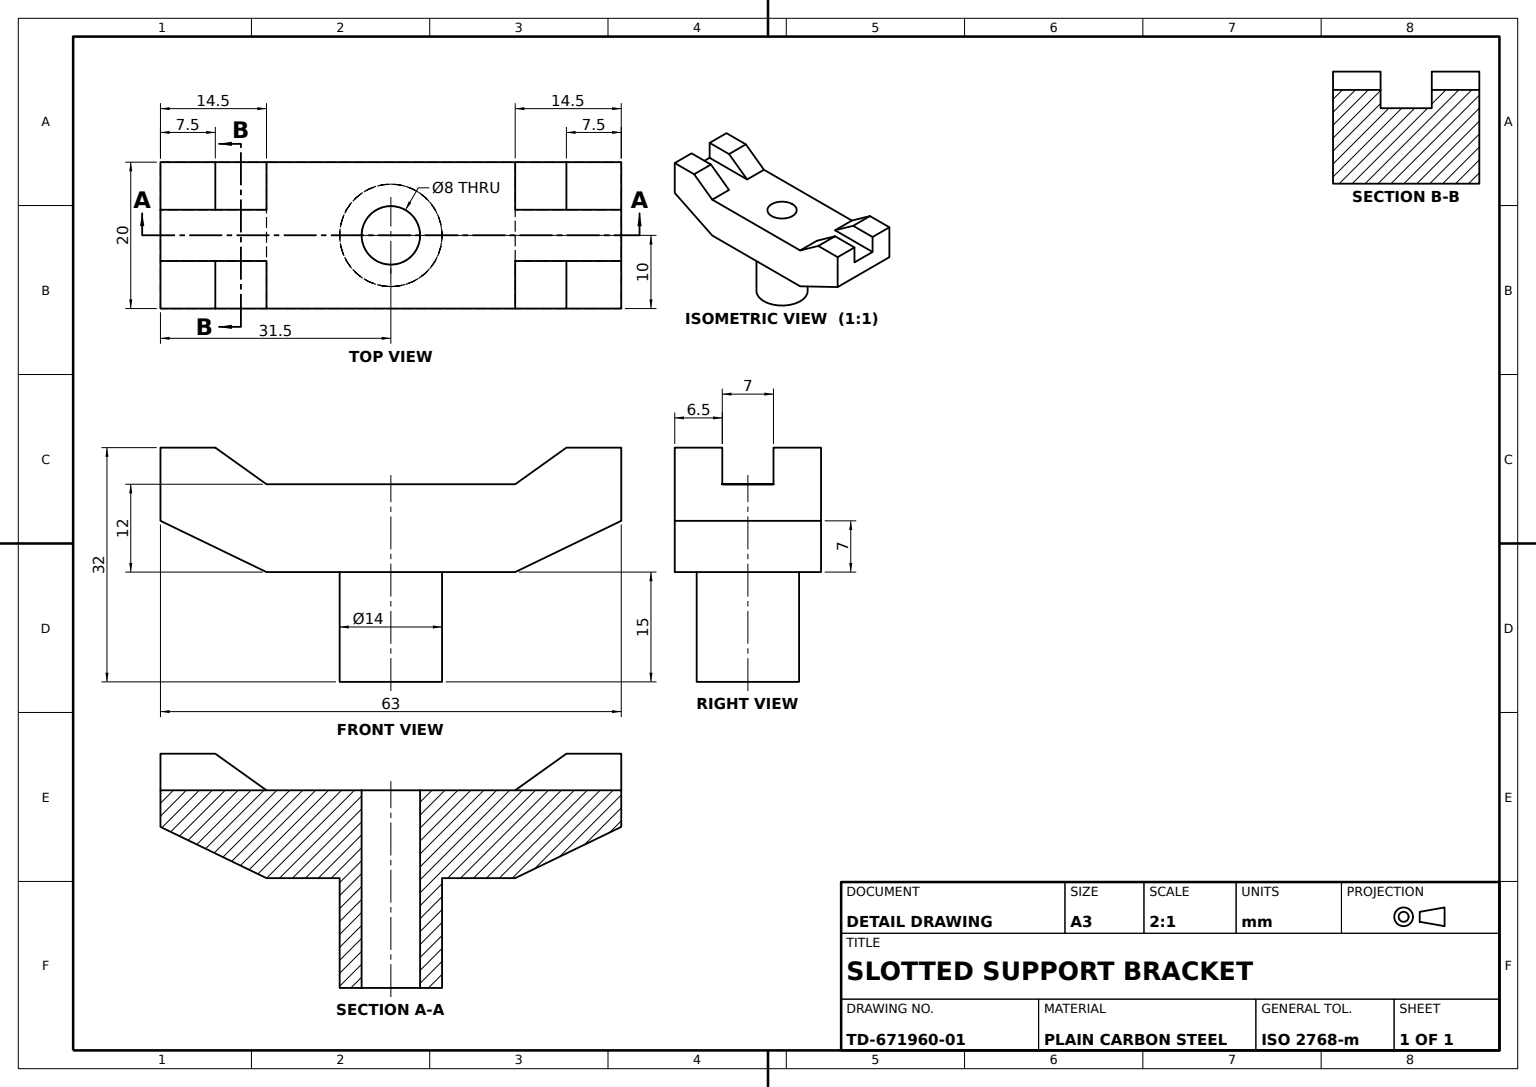
from build123d import *

# Parameters (mm, degrees)
BASE_BLOCK_DEPTH         = 20
END_LUGS_DEPTH           = 20
GUIDE_V_SLOT_DEPTH       = 63
LOCATING_PIN_SKETCH_14_R = 7
LOCATING_PIN_14_DEPTH    = 15
HOLE_SKETCH_8_R          = 4
HOLE_8_DEPTH             = 32


with BuildPart() as part:
    # Base Profile Sketch → Base Block (new body)
    with BuildSketch(Plane.XY):
        Polygon((0, 0), (63, 0), (63, -5), (48.5, -12), (31.5, -12), (14.5, -12), (0, -5), align=None)
    extrude(amount=BASE_BLOCK_DEPTH)

    # End Lugs Sketch → End Lugs (add)
    with BuildSketch(Plane.XY.offset(20)):
        Polygon((0, 0), (0, 5), (7.5, 5), (14.5, 0), align=None)
        Polygon((63, 0), (63, 5), (55.5, 5), (48.5, 0), align=None)
    extrude(amount=-END_LUGS_DEPTH)

    # Guide V-Slot Sketch → Guide V-Slot (cut)
    with BuildSketch(Plane.ZY):
        Polygon((10, 5), (6.5, 5), (6.5, 0), (13.5, 0), (13.5, 5), align=None)
    extrude(amount=-GUIDE_V_SLOT_DEPTH, mode=Mode.SUBTRACT)

    # Locating Pin Sketch Ø14 → Locating Pin Ø14 (add)
    with BuildSketch(Plane.XZ.offset(12)):
        with Locations(Location((31.5, 10, 0), (0, 0, 270))):
            Circle(LOCATING_PIN_SKETCH_14_R)
    extrude(amount=LOCATING_PIN_14_DEPTH)

    # Hole Sketch Ø8 → Hole Ø8 (cut)
    with BuildSketch(Plane(origin=(0, 0, 0), x_dir=(1, 0, 0), z_dir=(0, 1, 0))):
        with Locations(Location((31.5, -10, 0), (0, 0, 270))):
            Circle(HOLE_SKETCH_8_R)
    extrude(amount=-HOLE_8_DEPTH, mode=Mode.SUBTRACT)


solid = part.part
